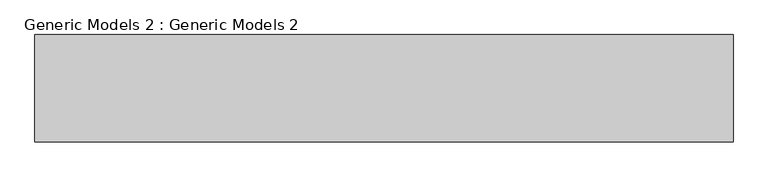
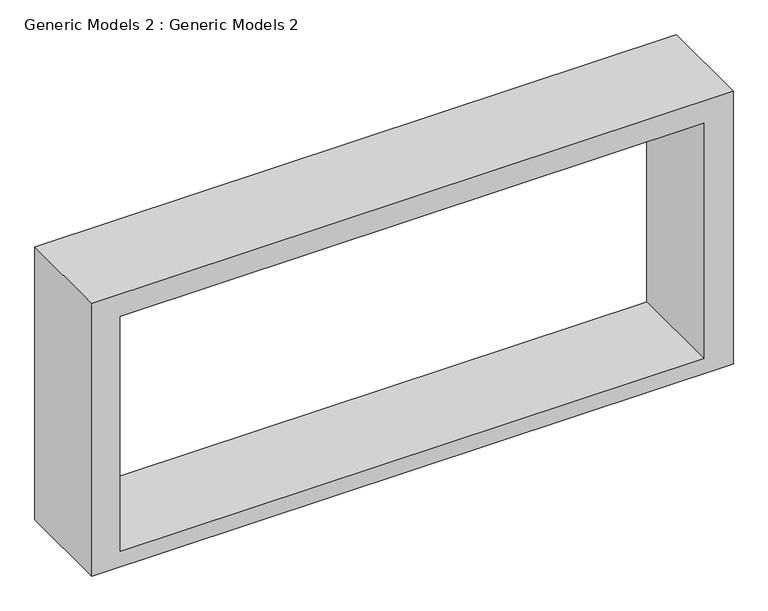
"""IFC4 building model written with IfcOpenShell, lengths in millimetres: proxy geometry, Generic Models 2 : Generic Models 2."""

from ifc_helpers import new_model, si_unit, frame, origin, place, context, project, spatial, polyline, outline, extrude, source, transform, mapped, element, save


def generic_models_2_generic_models_2_26ab94c5(model_context):
    return source(origin(), model_context, "Body", "SweptSolid", [
        extrude(outline(polyline([(6096.0, -4578.2831929), (6096.0, -10679.572128), (3352.8, -10679.572128), (3352.8, -4578.2831929), (6096.0, -4578.2831929)]), holes=[polyline([(5871.6595085, -10407.5831929), (5871.6595085, -4857.6831929), (3507.0931812, -4857.6831929), (3507.0931812, -10407.5831929), (5871.6595085, -10407.5831929)])]), frame((0.0, -11223.6654182, 0.0), z_axis=(0.0, 1.0, 0.0), x_axis=(0.0, 0.0, 1.0)), (0.0, 0.0, 1.0), 937.2061648),
    ])


if __name__ == "__main__":
    model = new_model("IFC4")
    model_context = context("Model", 3, world=origin())
    ifc_project = project(units=[si_unit("LENGTHUNIT", "METRE", prefix="MILLI")], contexts=[model_context])
    site = spatial("IfcSite", under=ifc_project)
    building = spatial("IfcBuilding", under=site)
    placement = place(None, origin())
    generic_models_2_generic_models_2_shape = generic_models_2_generic_models_2_26ab94c5(model_context)
    element("IfcBuildingElementProxy", 1, Name="Generic Models 2 : Generic Models 2", ObjectType="Generic Models 2 : Generic Models 2", at=placement, inside=building, context=model_context, shape_type="MappedRepresentation", body=[
        mapped(generic_models_2_generic_models_2_shape, transform((0.0, 0.0, 0.0), x_axis=(1.0, 0.0, 0.0), y_axis=(0.0, 1.0, 0.0), z_axis=(0.0, 0.0, 1.0))),
    ])
    save(model, "model.ifc")
